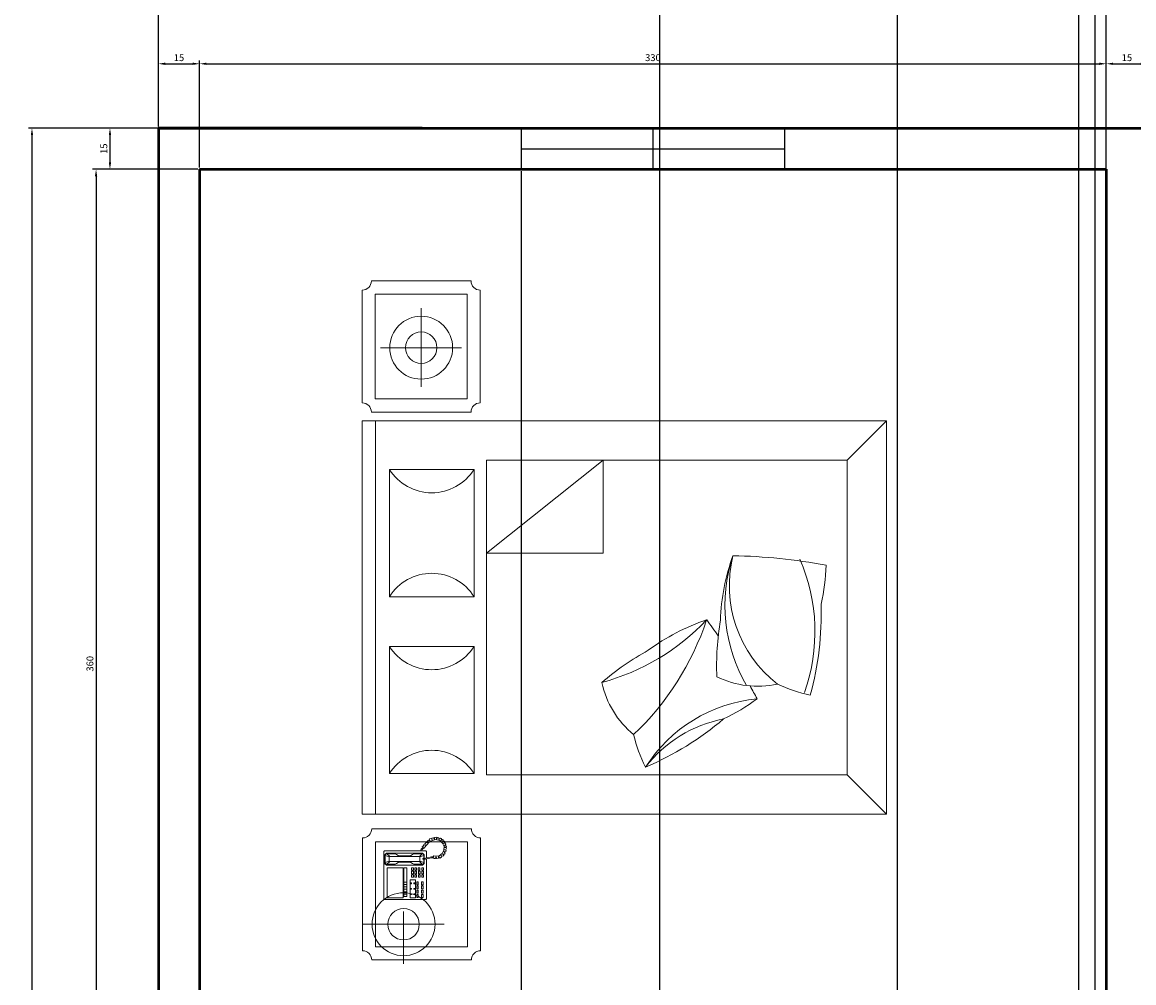
# Model space of a CAD drawing. Units: inches. Extents: x 604 to 3492, y -123 to 1737.
# Tile 8 of 20: x 628 to 1033, y 977 to 1326. Entities that reach past the tile are written whole.
import ezdxf

# ---------------------------------------------------------------- set-up
doc = ezdxf.new("R2010")
doc.units = ezdxf.units.IN
for name, color, linetype, lineweight in [('A-ANNO-DIMS', 2, 'Continuous', 18), ('A-FURN', 8, 'Continuous', 18), ('A-GLAZ', 4, 'Continuous', 25), ('A-WALL', 7, 'Continuous', 50)]:
    doc.layers.add(name, color=color, linetype=linetype, lineweight=lineweight)
doc.styles.get("Standard").update_dxf_attribs({"font": 'arial.ttf'})
doc.dimstyles.new('ISO-25', dxfattribs={"dimtxt": 2.5, "dimasz": 2.5, "dimexe": 1.25, "dimexo": 0.625, "dimtad": 1, "dimtxsty": 'Standard', "dimcen": 2.5, "dimadec": 0, "dimazin": 0, "dimtfac": 1, "dimtmove": 0, "dimatfit": 3, "dimfxl": 1, "dimarcsym": 0})

# ---------------------------------------------------------------- blocks, each defined once
blk = doc.blocks.new('A$C50B66110')
for p, q in [((0.0503, 1.9981), (0.4803, 1.9981)), ((0.1513, 1.6871), (0.1513, 1.9967)), ((0.5716, 1.9488), (0.5716, 2)), ((0.5716, 2), (2.0719, 2)), ((2.0719, 1.9488), (2.0719, 2)), ((2.5701, 1.9993), (2.1401, 1.9993)), ((0.0153, 1.9631), (0.0153, 1.5831)), ((0.5153, 1.9631), (0.5153, 1.5831)), ((2.1051, 1.9643), (2.1051, 1.5843)), ((2.6051, 1.9643), (2.6051, 1.5843)), ((0.0653, 1.9481), (0.0653, 1.5981)), ((0.0653, 1.9481), (0.4653, 1.9481)), ((0.4653, 1.9481), (0.4653, 1.5981)), ((2.0719, 1.9488), (0.5716, 1.9488)), ((0.5716, 1.9488), (0.5716, 0)), ((2.0719, 0), (2.0719, 1.9488)), ((2.1551, 1.9493), (2.1551, 1.5993)), ((2.5551, 1.9493), (2.1551, 1.9493)), ((2.3505, 1.62), (2.3505, 1.9295)), ((2.5551, 1.9493), (2.5551, 1.5993)), ((0.7257, 1.5725), (0.7257, 1.8954)), ((0.7257, 1.8954), (1.2113, 1.8954)), ((1.2113, 1.8954), (1.2113, 1.5725)), ((1.4007, 1.5725), (1.4007, 1.8954)), ((1.4007, 1.8954), (1.8863, 1.8954)), ((1.8863, 1.8954), (1.8863, 1.5725)), ((0, 1.8416), (0.2001, 1.8416)), ((2.5018, 1.7744), (2.2017, 1.7744)), ((0.0653, 1.5981), (0.4653, 1.5981)), ((1.2113, 1.5725), (0.7257, 1.5725)), ((1.8863, 1.5725), (1.4007, 1.5725)), ((2.5551, 1.5993), (2.1551, 1.5993)), ((0.0503, 1.5481), (0.4803, 1.5481)), ((2.5701, 1.5493), (2.1401, 1.5493)), ((1.5665, 1.5254), (1.5665, 1.0802)), ((1.5665, 1.5254), (1.9219, 1.0802)), ((1.9219, 1.0802), (1.5665, 1.0802)), ((0.5716, 0), (0.7216, 0.15)), ((2.0719, 0), (1.9219, 0.15)), ((0.5716, 0), (2.0719, 0))]:
    blk.add_line(p, q)
at = {"linetype": 'ByBlock'}
for p, q in [((0.2481, 1.9162), (0.2458, 1.9139)), ((0.2458, 1.9139), (0.2458, 1.7562)), ((0.2481, 1.9162), (0.4287, 1.9162)), ((0.3772, 1.9071), (0.3818, 1.9128)), ((0.3818, 1.9094), (0.3807, 1.9048)), ((0.3818, 1.9128), (0.4161, 1.9128)), ((0.3864, 1.9116), (0.3818, 1.9094)), ((0.3921, 1.8968), (0.3864, 1.9116)), ((0.3864, 1.9116), (0.4138, 1.9116)), ((0.4081, 1.8968), (0.4138, 1.9116)), ((0.4138, 1.9116), (0.4184, 1.9094)), ((0.4161, 1.9128), (0.4218, 1.9071)), ((0.4184, 1.9094), (0.4195, 1.9048)), ((0.4287, 1.9162), (0.4309, 1.9139)), ((0.4309, 1.9139), (0.4309, 1.7562)), ((0.2526, 1.9036), (0.2526, 1.8431)), ((0.3669, 1.9036), (0.2526, 1.9036)), ((0.3669, 1.8431), (0.3669, 1.9036)), ((0.3772, 1.7688), (0.3772, 1.9071)), ((0.3807, 1.9048), (0.3807, 1.8739)), ((0.3807, 1.9048), (0.3909, 1.8945)), ((0.3807, 1.8739), (0.3829, 1.8682)), ((0.3829, 1.8682), (0.3864, 1.8625)), ((0.3909, 1.8945), (0.3921, 1.8968)), ((0.3909, 1.8431), (0.3909, 1.8945)), ((0.4081, 1.8968), (0.3921, 1.8968)), ((0.4092, 1.8945), (0.4081, 1.8968)), ((0.4195, 1.9048), (0.4092, 1.8945)), ((0.4092, 1.8431), (0.4092, 1.8945)), ((0.4172, 1.8682), (0.4138, 1.8625)), ((0.4195, 1.8739), (0.4172, 1.8682)), ((0.4195, 1.9048), (0.4195, 1.8739)), ((0.4218, 1.9071), (0.4218, 1.7699)), ((0.2526, 1.8431), (0.3669, 1.8431)), ((0.2572, 1.8408), (0.2572, 1.8294)), ((0.3669, 1.8408), (0.2572, 1.8408)), ((0.2572, 1.8294), (0.3669, 1.8294)), ((0.2664, 1.8408), (0.2664, 1.8294)), ((0.2755, 1.8408), (0.2755, 1.8294)), ((0.2846, 1.8408), (0.2846, 1.8294)), ((0.2938, 1.8408), (0.2938, 1.8294)), ((0.3029, 1.8408), (0.3029, 1.8294)), ((0.3121, 1.8408), (0.3121, 1.8294)), ((0.3669, 1.8294), (0.3669, 1.8408)), ((0.3864, 1.8625), (0.3875, 1.8545)), ((0.3875, 1.8545), (0.3875, 1.8431)), ((0.3875, 1.8214), (0.3875, 1.8431)), ((0.3909, 1.8431), (0.3909, 1.7813)), ((0.4092, 1.8431), (0.4092, 1.7813)), ((0.4138, 1.8625), (0.4127, 1.8545)), ((0.4127, 1.8545), (0.4127, 1.8431)), ((0.4127, 1.8214), (0.4127, 1.8431)), ((0.3201, 1.8168), (0.2526, 1.8168)), ((0.2526, 1.8168), (0.2526, 1.7962)), ((0.2526, 1.7962), (0.3201, 1.7962)), ((0.2652, 1.7905), (0.2538, 1.7905)), ((0.2538, 1.7905), (0.2538, 1.7859)), ((0.2538, 1.7859), (0.2652, 1.7859)), ((0.2675, 1.8145), (0.2641, 1.8145)), ((0.2641, 1.8145), (0.2641, 1.8111)), ((0.2641, 1.8111), (0.2675, 1.8111)), ((0.2641, 1.8019), (0.2641, 1.7985)), ((0.2675, 1.8019), (0.2641, 1.8019)), ((0.2641, 1.7985), (0.2675, 1.7985)), ((0.2652, 1.7859), (0.2652, 1.7905)), ((0.2675, 1.8111), (0.2675, 1.8145)), ((0.2675, 1.7985), (0.2675, 1.8019)), ((0.2812, 1.7905), (0.2698, 1.7905)), ((0.2698, 1.7905), (0.2698, 1.7859)), ((0.2698, 1.7859), (0.2812, 1.7859)), ((0.2812, 1.7859), (0.2812, 1.7905)), ((0.2846, 1.8145), (0.2846, 1.8111)), ((0.2881, 1.8145), (0.2846, 1.8145)), ((0.2846, 1.8111), (0.2881, 1.8111)), ((0.2846, 1.8019), (0.2846, 1.7985)), ((0.2881, 1.8019), (0.2846, 1.8019)), ((0.2846, 1.7985), (0.2881, 1.7985)), ((0.2972, 1.7905), (0.2858, 1.7905)), ((0.2858, 1.7905), (0.2858, 1.7859)), ((0.2858, 1.7859), (0.2972, 1.7859)), ((0.2881, 1.8111), (0.2881, 1.8145)), ((0.2881, 1.7985), (0.2881, 1.8019)), ((0.2972, 1.7859), (0.2972, 1.7905)), ((0.3018, 1.7905), (0.3018, 1.7859)), ((0.3132, 1.7905), (0.3018, 1.7905)), ((0.3018, 1.7859), (0.3132, 1.7859)), ((0.3052, 1.8145), (0.3052, 1.8111)), ((0.3086, 1.8145), (0.3052, 1.8145)), ((0.3052, 1.8111), (0.3086, 1.8111)), ((0.3052, 1.8019), (0.3052, 1.7985)), ((0.3086, 1.8019), (0.3052, 1.8019)), ((0.3052, 1.7985), (0.3086, 1.7985)), ((0.3086, 1.8111), (0.3086, 1.8145)), ((0.3086, 1.7985), (0.3086, 1.8019)), ((0.3132, 1.7859), (0.3132, 1.7905)), ((0.3201, 1.7962), (0.3201, 1.8168)), ((0.3304, 1.8111), (0.3395, 1.8111)), ((0.3304, 1.8042), (0.3304, 1.8111)), ((0.3395, 1.8042), (0.3304, 1.8042)), ((0.3304, 1.7985), (0.3395, 1.7985)), ((0.3304, 1.7916), (0.3304, 1.7985)), ((0.3395, 1.7916), (0.3304, 1.7916)), ((0.3304, 1.7779), (0.3304, 1.7848)), ((0.3304, 1.7848), (0.3395, 1.7848)), ((0.3395, 1.8111), (0.3395, 1.8042)), ((0.3395, 1.7985), (0.3395, 1.7916)), ((0.3395, 1.7848), (0.3395, 1.7779)), ((0.3441, 1.8042), (0.3441, 1.8111)), ((0.3441, 1.8111), (0.3532, 1.8111)), ((0.3532, 1.8042), (0.3441, 1.8042)), ((0.3441, 1.7985), (0.3532, 1.7985)), ((0.3441, 1.7916), (0.3441, 1.7985)), ((0.3532, 1.7916), (0.3441, 1.7916)), ((0.3441, 1.7779), (0.3441, 1.7848)), ((0.3441, 1.7848), (0.3532, 1.7848)), ((0.3532, 1.8111), (0.3532, 1.8042)), ((0.3532, 1.7985), (0.3532, 1.7916)), ((0.3532, 1.7848), (0.3532, 1.7779)), ((0.3578, 1.8111), (0.3669, 1.8111)), ((0.3578, 1.8042), (0.3578, 1.8111)), ((0.3669, 1.8042), (0.3578, 1.8042)), ((0.3578, 1.7985), (0.3669, 1.7985)), ((0.3578, 1.7916), (0.3578, 1.7985)), ((0.3669, 1.7916), (0.3578, 1.7916)), ((0.3578, 1.7791), (0.3578, 1.7859)), ((0.3578, 1.7859), (0.3669, 1.7859)), ((0.3669, 1.8111), (0.3669, 1.8042)), ((0.3669, 1.7985), (0.3669, 1.7916)), ((0.3669, 1.7859), (0.3669, 1.7791)), ((0.3807, 1.8019), (0.3829, 1.8076)), ((0.3807, 1.7711), (0.3807, 1.8019)), ((0.3807, 1.7711), (0.3909, 1.7813)), ((0.3829, 1.8076), (0.3864, 1.8134)), ((0.3864, 1.8134), (0.3875, 1.8214)), ((0.3909, 1.7813), (0.3921, 1.7791)), ((0.4092, 1.7813), (0.4081, 1.7791)), ((0.4195, 1.7711), (0.4092, 1.7813)), ((0.4138, 1.8134), (0.4127, 1.8214)), ((0.4172, 1.8076), (0.4138, 1.8134)), ((0.4195, 1.8019), (0.4172, 1.8076)), ((0.4195, 1.7711), (0.4195, 1.8019)), ((0.2458, 1.7562), (0.2481, 1.7539)), ((0.4, 1.7539), (0.2481, 1.7539)), ((0.2538, 1.7665), (0.2538, 1.7733)), ((0.2538, 1.7733), (0.2652, 1.7733)), ((0.2652, 1.7665), (0.2538, 1.7665)), ((0.2652, 1.7733), (0.2652, 1.7665)), ((0.2698, 1.7665), (0.2698, 1.7733)), ((0.2698, 1.7733), (0.2812, 1.7733)), ((0.2812, 1.7665), (0.2698, 1.7665)), ((0.2812, 1.7733), (0.2812, 1.7665)), ((0.2858, 1.7665), (0.2858, 1.7733)), ((0.2858, 1.7733), (0.2972, 1.7733)), ((0.2972, 1.7665), (0.2858, 1.7665)), ((0.2972, 1.7733), (0.2972, 1.7665)), ((0.3018, 1.7733), (0.3132, 1.7733)), ((0.3018, 1.7665), (0.3018, 1.7733)), ((0.3132, 1.7665), (0.3018, 1.7665)), ((0.3132, 1.7733), (0.3132, 1.7665)), ((0.3395, 1.7779), (0.3304, 1.7779)), ((0.3304, 1.7722), (0.3395, 1.7722)), ((0.3304, 1.7653), (0.3304, 1.7722)), ((0.3395, 1.7653), (0.3304, 1.7653)), ((0.3395, 1.7722), (0.3395, 1.7653)), ((0.3532, 1.7779), (0.3441, 1.7779)), ((0.3441, 1.7722), (0.3532, 1.7722)), ((0.3441, 1.7653), (0.3441, 1.7722)), ((0.3532, 1.7653), (0.3441, 1.7653)), ((0.3532, 1.7722), (0.3532, 1.7653)), ((0.3669, 1.7791), (0.3578, 1.7791)), ((0.3578, 1.7653), (0.3578, 1.7722)), ((0.3578, 1.7722), (0.3669, 1.7722)), ((0.3669, 1.7653), (0.3578, 1.7653)), ((0.3669, 1.7722), (0.3669, 1.7653)), ((0.3829, 1.7631), (0.3772, 1.7688)), ((0.3818, 1.7665), (0.3807, 1.7711)), ((0.3864, 1.7642), (0.3818, 1.7665)), ((0.399, 1.7631), (0.3829, 1.7631)), ((0.3921, 1.7791), (0.3864, 1.7642)), ((0.3864, 1.7642), (0.399, 1.7642)), ((0.4081, 1.7791), (0.3921, 1.7791)), ((0.4024, 1.7676), (0.3989, 1.7676)), ((0.3989, 1.7676), (0.3991, 1.7578)), ((0.3991, 1.7578), (0.4019, 1.7462)), ((0.4019, 1.7462), (0.4047, 1.7353)), ((0.403, 1.7585), (0.4024, 1.7676)), ((0.4026, 1.7642), (0.4138, 1.7642)), ((0.4161, 1.7631), (0.4027, 1.7631)), ((0.4047, 1.7511), (0.403, 1.7585)), ((0.4287, 1.7539), (0.404, 1.7539)), ((0.4074, 1.7402), (0.4047, 1.7511)), ((0.4081, 1.7346), (0.4074, 1.7402)), ((0.4081, 1.7791), (0.4138, 1.7642)), ((0.4138, 1.7642), (0.4184, 1.7665)), ((0.4218, 1.7699), (0.4161, 1.7631)), ((0.4184, 1.7665), (0.4195, 1.7711)), ((0.4309, 1.7562), (0.4287, 1.7539)), ((0.4378, 1.7742), (0.4309, 1.7768)), ((0.4309, 1.7722), (0.436, 1.7708)), ((0.436, 1.7708), (0.4406, 1.7672)), ((0.441, 1.771), (0.4378, 1.7742)), ((0.4406, 1.7672), (0.4418, 1.7656)), ((0.4434, 1.7688), (0.441, 1.771)), ((0.4443, 1.7658), (0.4418, 1.7633)), ((0.4418, 1.7656), (0.4443, 1.7658)), ((0.4418, 1.7633), (0.4511, 1.7551)), ((0.4477, 1.7704), (0.4434, 1.7688)), ((0.4497, 1.7684), (0.4477, 1.7704)), ((0.4481, 1.765), (0.4497, 1.7684)), ((0.4509, 1.7672), (0.4481, 1.765)), ((0.4539, 1.764), (0.4509, 1.7672)), ((0.4511, 1.7551), (0.4662, 1.7422)), ((0.4515, 1.7573), (0.4539, 1.764)), ((0.4577, 1.7605), (0.4515, 1.7573)), ((0.463, 1.7555), (0.4577, 1.7605)), ((0.4618, 1.7482), (0.463, 1.7555)), ((0.467, 1.7515), (0.4618, 1.7482)), ((0.4664, 1.7418), (0.4741, 1.72)), ((0.4714, 1.7468), (0.467, 1.7515)), ((0.4696, 1.7418), (0.4714, 1.7468)), ((0.4766, 1.7425), (0.4697, 1.7418)), ((0.4787, 1.7356), (0.4766, 1.7425)), ((0.4026, 1.7254), (0.4021, 1.7198)), ((0.4021, 1.7198), (0.4088, 1.7187)), ((0.4088, 1.7187), (0.4023, 1.7147)), ((0.4023, 1.7147), (0.4028, 1.7085)), ((0.4051, 1.7279), (0.4026, 1.7254)), ((0.4028, 1.7085), (0.4102, 1.7078)), ((0.4102, 1.7078), (0.4037, 1.7027)), ((0.4037, 1.7027), (0.4067, 1.6974)), ((0.4047, 1.7353), (0.4044, 1.7293)), ((0.4044, 1.7293), (0.4051, 1.7279)), ((0.4067, 1.6974), (0.4137, 1.6988)), ((0.4079, 1.7286), (0.4081, 1.7346)), ((0.4121, 1.7256), (0.4079, 1.7286)), ((0.4137, 1.6988), (0.4104, 1.6923)), ((0.4111, 1.7203), (0.4121, 1.7256)), ((0.4123, 1.7057), (0.4111, 1.7203)), ((0.4211, 1.6946), (0.4123, 1.7057)), ((0.4708, 1.7027), (0.4606, 1.6927)), ((0.4741, 1.72), (0.4708, 1.7027)), ((0.4745, 1.6925), (0.4713, 1.6988)), ((0.4713, 1.6988), (0.478, 1.6967)), ((0.472, 1.733), (0.4787, 1.7356)), ((0.4794, 1.7332), (0.472, 1.733)), ((0.4743, 1.7075), (0.4815, 1.7073)), ((0.4798, 1.7013), (0.4743, 1.7075)), ((0.4761, 1.7233), (0.481, 1.7279)), ((0.4824, 1.7233), (0.4761, 1.7233)), ((0.4764, 1.7154), (0.4835, 1.7175)), ((0.4824, 1.7119), (0.4764, 1.7154)), ((0.478, 1.6967), (0.4798, 1.7013)), ((0.481, 1.7279), (0.4794, 1.7332)), ((0.4815, 1.7073), (0.4824, 1.7119)), ((0.4835, 1.7175), (0.4824, 1.7233)), ((0.4104, 1.6923), (0.4139, 1.6881)), ((0.4139, 1.6881), (0.4192, 1.692)), ((0.4192, 1.692), (0.4183, 1.6858)), ((0.4183, 1.6858), (0.4227, 1.683)), ((0.4333, 1.6881), (0.4211, 1.6946)), ((0.4227, 1.683), (0.4283, 1.6876)), ((0.4283, 1.6876), (0.4276, 1.68)), ((0.4276, 1.68), (0.4324, 1.6786)), ((0.4324, 1.6786), (0.4354, 1.6849)), ((0.4472, 1.6869), (0.4333, 1.6881)), ((0.4354, 1.6849), (0.4382, 1.6786)), ((0.4382, 1.6786), (0.4421, 1.6782)), ((0.4421, 1.6782), (0.4437, 1.6849)), ((0.4437, 1.6849), (0.4463, 1.6775)), ((0.4463, 1.6775), (0.4507, 1.6786)), ((0.4606, 1.6927), (0.4472, 1.6869)), ((0.4507, 1.6786), (0.4509, 1.6849)), ((0.4509, 1.6849), (0.4562, 1.6802)), ((0.4562, 1.6802), (0.4599, 1.6821)), ((0.4592, 1.689), (0.4641, 1.683)), ((0.4599, 1.6821), (0.4592, 1.689)), ((0.4641, 1.683), (0.4678, 1.6863)), ((0.465, 1.6925), (0.4715, 1.6897)), ((0.4678, 1.6863), (0.465, 1.6925)), ((0.4715, 1.6897), (0.4745, 1.6925)), ((0.7216, 1.5254), (1.9219, 1.5254)), ((0.7216, 1.5254), (0.7216, 0.15)), ((1.9219, 0.15), (1.9219, 1.5254)), ((0.7216, 0.15), (1.9219, 0.15))]:
    blk.add_line(p, q, dxfattribs=at)
for centre, radius in [((0.1513, 1.8416), 0.12), ((0.1513, 1.8416), 0.06), ((2.3505, 1.7744), 0.12), ((2.3505, 1.7744), 0.06)]:
    blk.add_circle(centre, radius)
for centre, radius, start, end in [((0.0153, 1.9981), 0.035, 270, 0), ((0.5153, 1.9981), 0.035, 180, 270), ((2.1051, 1.9993), 0.035, 270, 0), ((2.6051, 1.9993), 0.035, 180, 270), ((0.6244, 1.734), 0.1906, 302.1202, 57.8798), ((1.3126, 1.734), 0.1906, 122.1202, 237.8798), ((1.2994, 1.734), 0.1906, 302.1202, 57.8798), ((1.9876, 1.734), 0.1906, 122.1202, 237.8798), ((0.0153, 1.5481), 0.035, 0, 90), ((0.5153, 1.5481), 0.035, 90, 180), ((2.1051, 1.5493), 0.035, 0, 90), ((2.6051, 1.5493), 0.035, 90, 180), ((1.1502, 0.7366), 0.3575, 102.4782, 140.4625), ((0.328, 0.4368), 0.9879, 28.4971, 41.0566), ((1.9117, 1.3157), 0.8697, 195.336, 226.4193), ((0.9996, 0.4307), 0.548, 103.2034, 117.0362), ((1.656, 1.7093), 1.0798, 223.6306, 251.4288), ((0.4482, 0.4408), 0.5655, 5.3391, 57.6895), ((1.8226, 1.3753), 1.1652, 203.0642, 220.3209), ((0.4548, 0.5307), 0.4879, 10.6986, 52.6864), ((0.5648, 0.4378), 0.7874, 18.3527, 36.6851), ((-0.0179, 2.4352), 2.1977, 305.2966, 307.2418), ((1.4166, 0.4903), 0.3575, 154.0418, 192.0262), ((1.1403, -0.3401), 0.9879, 80.0607, 92.6202), ((1.5981, 0.9345), 0.734, 205.259, 216.9351), ((1.3672, 0.0075), 0.6085, 71.81, 120.1351), ((1.4431, 0.1219), 0.4774, 76.1849, 142.0017), ((1.2867, -0.154), 0.7874, 69.9163, 88.2487), ((-0.6401, 0.6314), 2.1977, 349.4884, 358.8054), ((-0.0179, 2.4352), 2.1977, 297.9248, 299.3793), ((1.5626, 0.1822), 0.548, 154.767, 168.5998), ((1.2678, 0.9611), 0.6885, 250.2936, 293.6414), ((1.3343, 1.4141), 1.1652, 254.6278, 271.8845), ((1.5399, 0.9642), 0.734, 256.8226, 268.4988)]:
    blk.add_arc(centre, radius, start, end)
blk = doc.blocks.new('*D10')
at = {"layer": 'A-ANNO-DIMS', "color": 0, "lineweight": -2, "transparency": 16777216}
for p, q in [((1023.01, 1273.33), (1023.01, 1312.37)), ((1025.51, 1311.12), (1035.51, 1311.12)), ((1038.01, 1273.33), (1038.01, 1312.37))]:
    blk.add_line(p, q, dxfattribs=at)
at = {"layer": 'A-ANNO-DIMS', "color": 0, "transparency": 16777216}
for points in [[(1025.51, 1311.54), (1025.51, 1310.71), (1023.01, 1311.12)], [(1035.51, 1311.54), (1035.51, 1310.71), (1038.01, 1311.12)]]:
    blk.add_solid(points, dxfattribs=at)
at = {"layer": 'Defpoints', "color": 0, "transparency": 16777216}
for p in [(1038.01, 1311.12), (1023.01, 1272.7), (1038.01, 1272.7)]:
    blk.add_point(p, dxfattribs=at)
at = {"layer": 'A-ANNO-DIMS', "color": 0, "transparency": 16777216, "insert": (1030.51, 1313.02), "char_height": 2.5, "attachment_point": 5}
blk.add_mtext('15', dxfattribs=at)
blk = doc.blocks.new('*D11')
at = {"layer": 'A-ANNO-DIMS', "color": 0, "lineweight": -2, "transparency": 16777216}
for p, q in [((693.01, 1273.33), (693.01, 1312.37)), ((695.51, 1311.12), (1020.51, 1311.12)), ((1023.01, 1273.33), (1023.01, 1312.37))]:
    blk.add_line(p, q, dxfattribs=at)
at = {"layer": 'A-ANNO-DIMS', "color": 0, "transparency": 16777216}
for points in [[(695.51, 1311.54), (695.51, 1310.71), (693.01, 1311.12)], [(1020.51, 1311.54), (1020.51, 1310.71), (1023.01, 1311.12)]]:
    blk.add_solid(points, dxfattribs=at)
at = {"layer": 'Defpoints', "color": 0, "transparency": 16777216}
for p in [(1023.01, 1311.12), (693.01, 1272.7), (1023.01, 1272.7)]:
    blk.add_point(p, dxfattribs=at)
at = {"layer": 'A-ANNO-DIMS', "color": 0, "transparency": 16777216, "insert": (858.01, 1313.02), "char_height": 2.5, "attachment_point": 5}
blk.add_mtext('330', dxfattribs=at)
blk = doc.blocks.new('*D12')
at = {"layer": 'A-ANNO-DIMS', "color": 0, "lineweight": -2, "transparency": 16777216}
for p, q in [((678.01, 1288.33), (678.01, 1312.37)), ((680.51, 1311.12), (690.51, 1311.12)), ((693.01, 1288.33), (693.01, 1312.37))]:
    blk.add_line(p, q, dxfattribs=at)
at = {"layer": 'A-ANNO-DIMS', "color": 0, "transparency": 16777216}
for points in [[(680.51, 1311.54), (680.51, 1310.71), (678.01, 1311.12)], [(690.51, 1311.54), (690.51, 1310.71), (693.01, 1311.12)]]:
    blk.add_solid(points, dxfattribs=at)
at = {"layer": 'Defpoints', "color": 0, "transparency": 16777216}
for p in [(693.01, 1311.12), (678.01, 1287.7), (693.01, 1287.7)]:
    blk.add_point(p, dxfattribs=at)
at = {"layer": 'A-ANNO-DIMS', "color": 0, "transparency": 16777216, "insert": (685.51, 1313.02), "char_height": 2.5, "attachment_point": 5}
blk.add_mtext('15', dxfattribs=at)
blk = doc.blocks.new('*D13')
at = {"layer": 'A-ANNO-DIMS', "color": 0, "lineweight": -2, "transparency": 16777216}
for p, q in [((678.01, 1288.33), (678.01, 1383.12)), ((680.51, 1381.87), (1350.51, 1381.87)), ((1353.01, 1288.33), (1353.01, 1383.12))]:
    blk.add_line(p, q, dxfattribs=at)
at = {"layer": 'A-ANNO-DIMS', "color": 0, "transparency": 16777216}
for points in [[(680.51, 1382.29), (680.51, 1381.46), (678.01, 1381.87)], [(1350.51, 1382.29), (1350.51, 1381.46), (1353.01, 1381.87)]]:
    blk.add_solid(points, dxfattribs=at)
at = {"layer": 'Defpoints', "color": 0, "transparency": 16777216}
for p in [(1353.01, 1381.87), (678.01, 1287.7), (1353.01, 1287.7)]:
    blk.add_point(p, dxfattribs=at)
at = {"layer": 'A-ANNO-DIMS', "color": 0, "transparency": 16777216, "insert": (1015.51, 1383.78), "char_height": 2.5, "attachment_point": 5}
blk.add_mtext('675', dxfattribs=at)
blk = doc.blocks.new('*D21')
at = {"layer": 'A-ANNO-DIMS', "color": 0, "lineweight": -2, "transparency": 16777216}
for p, q in [((692.39, 1287.7), (659.14, 1287.7)), ((660.39, 1285.2), (660.39, 1275.2)), ((692.39, 1272.7), (659.14, 1272.7))]:
    blk.add_line(p, q, dxfattribs=at)
at = {"layer": 'A-ANNO-DIMS', "color": 0, "transparency": 16777216}
for points in [[(659.98, 1285.2), (660.81, 1285.2), (660.39, 1287.7)], [(659.98, 1275.2), (660.81, 1275.2), (660.39, 1272.7)]]:
    blk.add_solid(points, dxfattribs=at)
at = {"layer": 'Defpoints', "color": 0, "transparency": 16777216}
for p in [(693.01, 1287.7), (660.39, 1272.7), (693.01, 1272.7)]:
    blk.add_point(p, dxfattribs=at)
at = {"layer": 'A-ANNO-DIMS', "color": 0, "transparency": 16777216, "insert": (658.49, 1280.2), "char_height": 2.5, "attachment_point": 5, "rotation": 90}
blk.add_mtext('15', dxfattribs=at)
blk = doc.blocks.new('*D22')
at = {"layer": 'A-ANNO-DIMS', "color": 0, "lineweight": -2, "transparency": 16777216}
for p, q in [((692.39, 1272.7), (654.09, 1272.7)), ((655.34, 1270.2), (655.34, 915.2)), ((692.39, 912.7), (654.09, 912.7))]:
    blk.add_line(p, q, dxfattribs=at)
at = {"layer": 'A-ANNO-DIMS', "color": 0, "transparency": 16777216}
for points in [[(654.92, 1270.2), (655.75, 1270.2), (655.34, 1272.7)], [(654.92, 915.2), (655.75, 915.2), (655.34, 912.7)]]:
    blk.add_solid(points, dxfattribs=at)
at = {"layer": 'Defpoints', "color": 0, "transparency": 16777216}
for p in [(693.01, 1272.7), (655.34, 912.7), (693.01, 912.7)]:
    blk.add_point(p, dxfattribs=at)
at = {"layer": 'A-ANNO-DIMS', "color": 0, "transparency": 16777216, "insert": (653.44, 1092.7), "char_height": 2.5, "attachment_point": 5, "rotation": 90}
blk.add_mtext('360', dxfattribs=at)
blk = doc.blocks.new('*D37')
at = {"layer": 'A-ANNO-DIMS', "color": 0, "lineweight": -2, "transparency": 16777216}
for p, q in [((677.39, 1287.7), (630.76, 1287.7)), ((632.01, 1285.2), (632.01, 290.2)), ((677.39, 287.7), (630.76, 287.7))]:
    blk.add_line(p, q, dxfattribs=at)
at = {"layer": 'A-ANNO-DIMS', "color": 0, "transparency": 16777216}
for points in [[(631.59, 1285.2), (632.42, 1285.2), (632.01, 1287.7)], [(631.59, 290.2), (632.42, 290.2), (632.01, 287.7)]]:
    blk.add_solid(points, dxfattribs=at)
at = {"layer": 'Defpoints', "color": 0, "transparency": 16777216}
for p in [(678.01, 1287.7), (632.01, 287.7), (678.01, 287.7)]:
    blk.add_point(p, dxfattribs=at)
at = {"layer": 'A-ANNO-DIMS', "color": 0, "transparency": 16777216, "insert": (630.1, 787.7), "char_height": 2.5, "attachment_point": 5, "rotation": 90}
blk.add_mtext('1000', dxfattribs=at)
blk = doc.blocks.new('WIN-96')
for p, q in [((15, 96), (0, 96)), ((7.5, 96), (7.5, 0)), ((15, 96), (15, 0)), ((15, 48), (0, 48))]:
    blk.add_line(p, q)
blk.add_lwpolyline([(0, 96), (0, 0), (15, 0), (15, 96)], close=True)
blk = doc.blocks.new('*D85')
at = {"layer": 'A-ANNO-DIMS', "color": 0, "lineweight": -2, "transparency": 16777216}
for p, q in [((693.01, 1272.08), (693.01, 67.77)), ((810.01, 1272.08), (810.01, 67.77)), ((695.51, 69.02), (807.51, 69.02))]:
    blk.add_line(p, q, dxfattribs=at)
at = {"layer": 'A-ANNO-DIMS', "color": 0, "transparency": 16777216}
for points in [[(695.51, 69.44), (695.51, 68.61), (693.01, 69.02)], [(807.51, 69.44), (807.51, 68.61), (810.01, 69.02)]]:
    blk.add_solid(points, dxfattribs=at)
at = {"layer": 'Defpoints', "color": 0, "transparency": 16777216}
for p in [(693.01, 1272.7), (810.01, 1272.7), (810.01, 69.02)]:
    blk.add_point(p, dxfattribs=at)
at = {"layer": 'A-ANNO-DIMS', "color": 0, "transparency": 16777216, "insert": (751.51, 70.9), "char_height": 2.5, "attachment_point": 5}
blk.add_mtext('117', dxfattribs=at)
blk = doc.blocks.new('*D90')
at = {"layer": 'A-ANNO-DIMS', "color": 0, "lineweight": -2, "transparency": 16777216}
for p, q in [((1019.01, 423.33), (1019.01, 1359.9)), ((1023.01, 423.33), (1023.01, 1359.9)), ((1016.51, 1358.65), (1014.01, 1358.65)), ((1023.01, 1358.65), (1019.01, 1358.65)), ((1025.51, 1358.65), (1028.01, 1358.65))]:
    blk.add_line(p, q, dxfattribs=at)
at = {"layer": 'A-ANNO-DIMS', "color": 0, "transparency": 16777216}
for points in [[(1016.51, 1359.07), (1016.51, 1358.23), (1019.01, 1358.65)], [(1025.51, 1359.07), (1025.51, 1358.23), (1023.01, 1358.65)]]:
    blk.add_solid(points, dxfattribs=at)
at = {"layer": 'Defpoints', "color": 0, "transparency": 16777216}
for p in [(1019.01, 1358.65), (1019.01, 422.7), (1023.01, 422.7)]:
    blk.add_point(p, dxfattribs=at)
at = {"layer": 'A-ANNO-DIMS', "color": 0, "transparency": 16777216, "insert": (1021.01, 1360.53), "char_height": 2.5, "attachment_point": 5}
blk.add_mtext('4', dxfattribs=at)
blk = doc.blocks.new('*D91')
at = {"layer": 'A-ANNO-DIMS', "color": 0, "lineweight": -2, "transparency": 16777216}
for p, q in [((860.51, 408.33), (860.51, 1359.9)), ((947.01, 408.33), (947.01, 1359.9)), ((863.01, 1358.65), (944.51, 1358.65))]:
    blk.add_line(p, q, dxfattribs=at)
at = {"layer": 'A-ANNO-DIMS', "color": 0, "transparency": 16777216}
for points in [[(863.01, 1359.07), (863.01, 1358.23), (860.51, 1358.65)], [(944.51, 1359.07), (944.51, 1358.23), (947.01, 1358.65)]]:
    blk.add_solid(points, dxfattribs=at)
at = {"layer": 'Defpoints', "color": 0, "transparency": 16777216}
for p in [(947.01, 1358.65), (860.51, 407.7), (947.01, 407.7)]:
    blk.add_point(p, dxfattribs=at)
at = {"layer": 'A-ANNO-DIMS', "color": 0, "transparency": 16777216, "insert": (903.76, 1360.55), "char_height": 2.5, "attachment_point": 5}
blk.add_mtext('86.5', dxfattribs=at)
blk = doc.blocks.new('*D99')
at = {"layer": 'A-ANNO-DIMS', "color": 0, "lineweight": -2, "transparency": 16777216}
for p, q in [((1013.01, 898.33), (1013.01, 1359.9)), ((1023.01, 913.33), (1023.01, 1359.9)), ((1015.51, 1358.65), (1020.51, 1358.65))]:
    blk.add_line(p, q, dxfattribs=at)
at = {"layer": 'A-ANNO-DIMS', "color": 0, "transparency": 16777216}
for points in [[(1015.51, 1359.07), (1015.51, 1358.23), (1013.01, 1358.65)], [(1020.51, 1359.07), (1020.51, 1358.23), (1023.01, 1358.65)]]:
    blk.add_solid(points, dxfattribs=at)
at = {"layer": 'Defpoints', "color": 0, "transparency": 16777216}
for p in [(1023.01, 1358.65), (1023.01, 912.7), (1013.01, 897.7)]:
    blk.add_point(p, dxfattribs=at)
at = {"layer": 'A-ANNO-DIMS', "color": 0, "transparency": 16777216, "insert": (1018.01, 1360.55), "char_height": 2.5, "attachment_point": 5}
blk.add_mtext('10', dxfattribs=at)

msp = doc.modelspace()

# ---------------------------------------------------------------- linework, layer by layer
at = {"layer": 'A-WALL'}
for p, q in [((678.0111, 1287.7004), (1353.0111, 1287.7004)), ((678.0111, 1287.7004), (678.0111, 287.7004)), ((678.0111, 1287.7004), (774.0111, 1287.7004)), ((678.0111, 1287.7004), (678.0111, 1272.7004)), ((693.0111, 1272.7004), (1023.0111, 1272.7004)), ((693.0111, 1272.7004), (693.0111, 912.7004)), ((693.0111, 1272.7004), (1023.0111, 1272.7004)), ((1023.0111, 1272.7004), (1023.0111, 912.7004))]:
    msp.add_line(p, q, dxfattribs=at)
for points in [[(774.0111, 1287.7004), (678.0111, 1287.7004), (678.0111, 1272.7004)], [(693.0111, 1272.7004), (774.0111, 1272.7004)]]:
    msp.add_lwpolyline(points, dxfattribs=at)

# ---------------------------------------------------------------- block references
at = {"layer": 'A-FURN', "xscale": 95.4379570199766, "yscale": 95.4379570199766, "zscale": 95.4379570199766, "rotation": 90}
msp.add_blockref('A$C50B66110', (943.0058, 983.438), dxfattribs=at)
at = {"layer": 'A-GLAZ', "rotation": 89.99999999999908}
msp.add_blockref('WIN-96', (906.0111, 1272.7004), dxfattribs=at)

# ---------------------------------------------------------------- dimensions: what is measured, and where the dimension line sits
at = {"layer": 'A-ANNO-DIMS'}
for base, p1, p2, override, picture, middle in [((1353.0111, 1381.8744), (678.0111, 1287.7004), (1353.0111, 1287.7004), {"dimclrd": 0, "dimclre": 0, "dimclrt": 0}, '*D13', (1015.5111, 1383.7759)), ((947.0111, 1358.6504), (860.5111, 407.7004), (947.0111, 407.7004), {"dimdec": 1, "dimlfac": 1, "dimrnd": 0, "dimzin": 0, "dimdsep": 46, "dimlunit": 2}, '*D91', (903.7611, 1360.5519)), ((1023.0111, 1358.6504), (1013.0111, 897.7004), (1023.0111, 912.7004), {"dimdec": 0, "dimlfac": 1, "dimrnd": 0, "dimzin": 0, "dimdsep": 46, "dimlunit": 2}, '*D99', (1018.0111, 1360.5519)), ((1019.0111, 1358.6504), (1023.0111, 422.7004), (1019.0111, 422.7004), {"dimdec": 0, "dimlfac": 1, "dimrnd": 0, "dimzin": 0, "dimdsep": 46, "dimlunit": 2}, '*D90', (1021.0111, 1360.5254)), ((693.0111, 1311.1217), (678.0111, 1287.7004), (693.0111, 1287.7004), {"dimclrd": 0, "dimclre": 0, "dimclrt": 0}, '*D12', (685.5111, 1313.0232)), ((1023.0111, 1311.1217), (693.0111, 1272.7004), (1023.0111, 1272.7004), {"dimclrd": 0, "dimclre": 0, "dimclrt": 0}, '*D11', (858.0111, 1313.024)), ((1038.0111, 1311.1217), (1023.0111, 1272.7004), (1038.0111, 1272.7004), {"dimclrd": 0, "dimclre": 0, "dimclrt": 0}, '*D10', (1030.5111, 1313.0232)), ((810.0111, 69.0242), (693.0111, 1272.7004), (810.0111, 1272.7004), {"dimdec": 0, "dimlfac": 1, "dimrnd": 0, "dimzin": 0, "dimdsep": 46, "dimlunit": 2}, '*D85', (751.5111, 70.9043))]:
    dim = msp.add_linear_dim(base=base, p1=p1, p2=p2, dimstyle='ISO-25', override=override, dxfattribs=at)
    dim.commit()
    dim.dimension.update_dxf_attribs({"geometry": picture, "text_midpoint": middle})
for base, p1, p2, picture, middle in [((632.0054, 287.7004), (678.0111, 1287.7004), (678.0111, 287.7004), '*D37', (630.104, 787.7004)), ((660.3934, 1272.7004), (693.0111, 1287.7004), (693.0111, 1272.7004), '*D21', (658.492, 1280.2004)), ((655.3379, 912.7004), (693.0111, 1272.7004), (693.0111, 912.7004), '*D22', (653.4356, 1092.7004))]:
    dim = msp.add_linear_dim(base=base, p1=p1, p2=p2, angle=90, dimstyle='ISO-25', override={"dimclrd": 0, "dimclre": 0, "dimclrt": 0}, dxfattribs=at)
    dim.commit()
    dim.dimension.update_dxf_attribs({"geometry": picture, "text_midpoint": middle})

doc.saveas('drawing.dxf')
